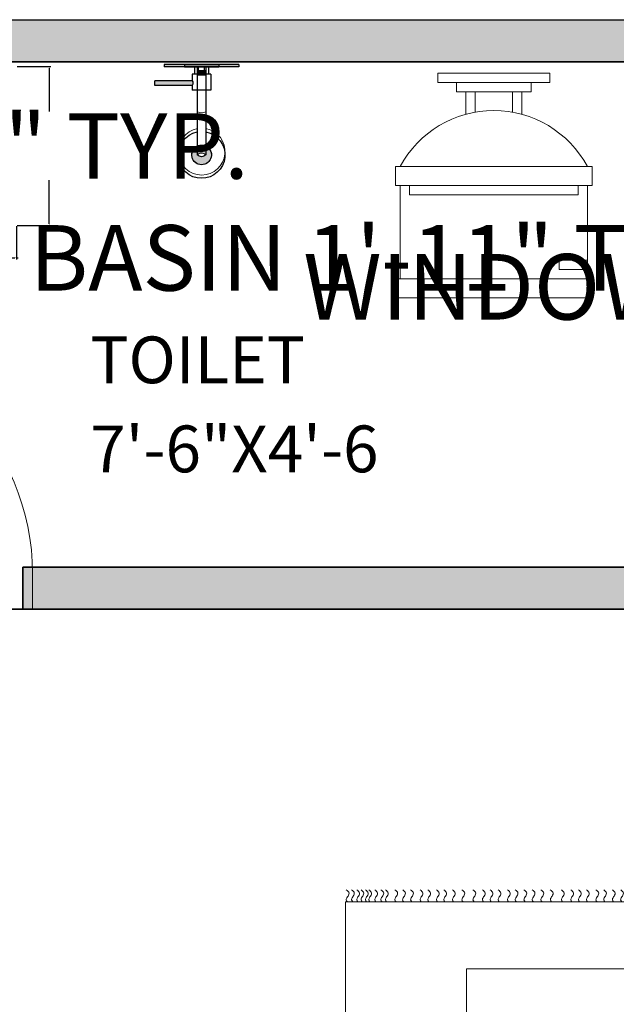
# Model space of a CAD drawing. Units: inches. Extents: x 0 to 4258, y 0 to 3769.
# Tile 22 of 30: x 3708 to 3772, y 3552 to 3657. Entities that reach past the tile are written whole.
import ezdxf

# ---------------------------------------------------------------- set-up
doc = ezdxf.new("R2010")
doc.units = ezdxf.units.IN
doc.header["$MEASUREMENT"] = 0
doc.layers.get('0').update_dxf_attribs({"color": 16})
for name, color, linetype, lineweight in [('A-ANNO-DIMS', 250, 'Continuous', 18), ('A-AREA-IDEN', 250, 'Continuous', 18), ('A-FLOR-FIXT', 250, 'Continuous', 18), ('A-WALL-PATT', 16, 'Continuous', 13), ('C-PROP', 150, 'Continuous', 25), ('doors', 250, 'Continuous', 18), ('furniture', 13, 'Continuous', 18), ('walls', 251, 'Continuous', 35)]:
    doc.layers.add(name, color=color, linetype=linetype, lineweight=lineweight)
doc.layers.add('PLUMBING FIXTURES', color=250, linetype='Continuous')
doc.styles.get("Standard").update_dxf_attribs({"font": 'arial.ttf'})
doc.dimstyles.get("Standard").update_dxf_attribs({"dimtxt": 7, "dimasz": 0.18, "dimexe": 0.18, "dimexo": 0.0625, "dimgap": 0.09, "dimtad": 0, "dimtih": 1, "dimtoh": 1, "dimzin": 0, "dimdsep": 46, "dimlunit": 3, "dimtxsty": 'Standard', "dimcen": 0.09, "dimadec": 0, "dimazin": 0, "dimtfac": 1, "dimtofl": 0, "dimtmove": 0, "dimatfit": 3, "dimfxl": 1, "dimtolj": 1, "dimtzin": 0, "dimarcsym": 0})

# ---------------------------------------------------------------- blocks, each defined once
blk = doc.blocks.new('CARPET')
at = {"layer": 'furniture'}
for p, q in [((-51.53, -98.11), (-51.53, -55.12)), ((-51.53, -55.12), (-41.27, -55.12)), ((36, -55.12), (51.55, -55.12)), ((51.55, -55.12), (51.55, -98.11)), ((51.55, -98.11), (-51.53, -98.11))]:
    blk.add_line(p, q, dxfattribs=at)
for points, knots in [([(-53.37, -55.99), (-53.22, -55.8), (-52.9, -55.41), (-52.34, -55.8), (-51.89, -56.08), (-51.65, -55.91), (-51.53, -55.83)], [0, 0, 0, 0, 0.653278, 1.290138, 1.740457, 2.114451, 2.114451, 2.114451, 2.114451]), ([(53.37, -55.99), (53.22, -55.8), (52.9, -55.41), (52.34, -55.8), (51.89, -56.08), (51.65, -55.91), (51.53, -55.83)], [0, 0, 0, 0, 0.653278, 1.290138, 1.740457, 2.114451, 2.114451, 2.114451, 2.114451]), ([(-53.37, -57.26), (-53.22, -57.07), (-52.9, -56.67), (-52.34, -57.07), (-51.89, -57.35), (-51.65, -57.17), (-51.53, -57.1)], [0, 0, 0, 0, 0.653278, 1.290138, 1.740457, 2.114451, 2.114451, 2.114451, 2.114451]), ([(53.37, -57.26), (53.22, -57.07), (52.9, -56.67), (52.34, -57.07), (51.89, -57.35), (51.65, -57.17), (51.53, -57.1)], [0, 0, 0, 0, 0.653278, 1.290138, 1.740457, 2.114451, 2.114451, 2.114451, 2.114451]), ([(-53.37, -58.59), (-53.22, -58.4), (-52.9, -58.01), (-52.34, -58.4), (-51.89, -58.68), (-51.65, -58.5), (-51.53, -58.43)], [0, 0, 0, 0, 0.653278, 1.290138, 1.740457, 2.114451, 2.114451, 2.114451, 2.114451]), ([(53.37, -58.59), (53.22, -58.4), (52.9, -58.01), (52.34, -58.4), (51.89, -58.68), (51.65, -58.5), (51.53, -58.43)], [0, 0, 0, 0, 0.653278, 1.290138, 1.740457, 2.114451, 2.114451, 2.114451, 2.114451]), ([(-53.37, -59.78), (-53.22, -59.58), (-52.9, -59.19), (-52.34, -59.58), (-51.89, -59.86), (-51.65, -59.69), (-51.53, -59.61)], [0, 0, 0, 0, 0.653278, 1.290138, 1.740457, 2.114451, 2.114451, 2.114451, 2.114451]), ([(53.37, -59.78), (53.22, -59.58), (52.9, -59.19), (52.34, -59.58), (51.89, -59.86), (51.65, -59.69), (51.53, -59.61)], [0, 0, 0, 0, 0.653278, 1.290138, 1.740457, 2.114451, 2.114451, 2.114451, 2.114451]), ([(-53.37, -61.22), (-53.22, -61.02), (-52.9, -60.63), (-52.34, -61.02), (-51.89, -61.3), (-51.65, -61.13), (-51.53, -61.05)], [0, 0, 0, 0, 0.653278, 1.290138, 1.740457, 2.114451, 2.114451, 2.114451, 2.114451]), ([(53.37, -61.22), (53.22, -61.02), (52.9, -60.63), (52.34, -61.02), (51.89, -61.3), (51.65, -61.13), (51.53, -61.05)], [0, 0, 0, 0, 0.653278, 1.290138, 1.740457, 2.114451, 2.114451, 2.114451, 2.114451]), ([(-53.37, -62.44), (-53.22, -62.25), (-52.9, -61.86), (-52.34, -62.25), (-51.89, -62.53), (-51.65, -62.36), (-51.53, -62.28)], [0, 0, 0, 0, 0.653278, 1.290138, 1.740457, 2.114451, 2.114451, 2.114451, 2.114451]), ([(-53.37, -63.63), (-53.22, -63.43), (-52.9, -63.04), (-52.34, -63.43), (-51.89, -63.72), (-51.65, -63.54), (-51.53, -63.46)], [0, 0, 0, 0, 0.653278, 1.290138, 1.740457, 2.114451, 2.114451, 2.114451, 2.114451]), ([(53.37, -62.44), (53.22, -62.25), (52.9, -61.86), (52.34, -62.25), (51.89, -62.53), (51.65, -62.36), (51.53, -62.28)], [0, 0, 0, 0, 0.653278, 1.290138, 1.740457, 2.114451, 2.114451, 2.114451, 2.114451]), ([(53.37, -63.63), (53.22, -63.43), (52.9, -63.04), (52.34, -63.43), (51.89, -63.72), (51.65, -63.54), (51.53, -63.46)], [0, 0, 0, 0, 0.653278, 1.290138, 1.740457, 2.114451, 2.114451, 2.114451, 2.114451]), ([(-53.37, -65.07), (-53.22, -64.87), (-52.9, -64.48), (-52.34, -64.87), (-51.89, -65.15), (-51.65, -64.98), (-51.53, -64.9)], [0, 0, 0, 0, 0.653278, 1.290138, 1.740457, 2.114451, 2.114451, 2.114451, 2.114451]), ([(53.37, -65.07), (53.22, -64.87), (52.9, -64.48), (52.34, -64.87), (51.89, -65.15), (51.65, -64.98), (51.53, -64.9)], [0, 0, 0, 0, 0.653278, 1.290138, 1.740457, 2.114451, 2.114451, 2.114451, 2.114451]), ([(-53.37, -66.76), (-53.22, -66.56), (-52.9, -66.17), (-52.34, -66.56), (-51.89, -66.84), (-51.65, -66.67), (-51.53, -66.59)], [0, 0, 0, 0, 0.653278, 1.290138, 1.740457, 2.114451, 2.114451, 2.114451, 2.114451]), ([(-53.37, -68.2), (-53.22, -68), (-52.9, -67.61), (-52.34, -68), (-51.89, -68.28), (-51.65, -68.11), (-51.53, -68.03)], [0, 0, 0, 0, 0.653278, 1.290138, 1.740457, 2.114451, 2.114451, 2.114451, 2.114451]), ([(53.37, -66.76), (53.22, -66.56), (52.9, -66.17), (52.34, -66.56), (51.89, -66.84), (51.65, -66.67), (51.53, -66.59)], [0, 0, 0, 0, 0.653278, 1.290138, 1.740457, 2.114451, 2.114451, 2.114451, 2.114451]), ([(53.37, -68.2), (53.22, -68), (52.9, -67.61), (52.34, -68), (51.89, -68.28), (51.65, -68.11), (51.53, -68.03)], [0, 0, 0, 0, 0.653278, 1.290138, 1.740457, 2.114451, 2.114451, 2.114451, 2.114451]), ([(-53.37, -69.53), (-53.22, -69.33), (-52.9, -68.94), (-52.34, -69.33), (-51.89, -69.61), (-51.65, -69.44), (-51.53, -69.36)], [0, 0, 0, 0, 0.653278, 1.290138, 1.740457, 2.114451, 2.114451, 2.114451, 2.114451]), ([(53.37, -69.53), (53.22, -69.33), (52.9, -68.94), (52.34, -69.33), (51.89, -69.61), (51.65, -69.44), (51.53, -69.36)], [0, 0, 0, 0, 0.653278, 1.290138, 1.740457, 2.114451, 2.114451, 2.114451, 2.114451]), ([(-53.37, -70.79), (-53.22, -70.6), (-52.9, -70.21), (-52.34, -70.6), (-51.89, -70.88), (-51.65, -70.7), (-51.53, -70.63)], [0, 0, 0, 0, 0.653278, 1.290138, 1.740457, 2.114451, 2.114451, 2.114451, 2.114451]), ([(53.37, -70.79), (53.22, -70.6), (52.9, -70.21), (52.34, -70.6), (51.89, -70.88), (51.65, -70.7), (51.53, -70.63)], [0, 0, 0, 0, 0.653278, 1.290138, 1.740457, 2.114451, 2.114451, 2.114451, 2.114451]), ([(-53.37, -72.12), (-53.22, -71.93), (-52.9, -71.54), (-52.34, -71.93), (-51.89, -72.21), (-51.65, -72.04), (-51.53, -71.96)], [0, 0, 0, 0, 0.653278, 1.290138, 1.740457, 2.114451, 2.114451, 2.114451, 2.114451]), ([(53.37, -72.12), (53.22, -71.93), (52.9, -71.54), (52.34, -71.93), (51.89, -72.21), (51.65, -72.04), (51.53, -71.96)], [0, 0, 0, 0, 0.653278, 1.290138, 1.740457, 2.114451, 2.114451, 2.114451, 2.114451]), ([(-53.37, -73.31), (-53.22, -73.11), (-52.9, -72.72), (-52.34, -73.11), (-51.89, -73.4), (-51.65, -73.22), (-51.53, -73.14)], [0, 0, 0, 0, 0.653278, 1.290138, 1.740457, 2.114451, 2.114451, 2.114451, 2.114451]), ([(53.37, -73.31), (53.22, -73.11), (52.9, -72.72), (52.34, -73.11), (51.89, -73.4), (51.65, -73.22), (51.53, -73.14)], [0, 0, 0, 0, 0.653278, 1.290138, 1.740457, 2.114451, 2.114451, 2.114451, 2.114451]), ([(-53.37, -74.75), (-53.22, -74.55), (-52.9, -74.16), (-52.34, -74.55), (-51.89, -74.83), (-51.65, -74.66), (-51.53, -74.58)], [0, 0, 0, 0, 0.653278, 1.290138, 1.740457, 2.114451, 2.114451, 2.114451, 2.114451]), ([(53.37, -74.75), (53.22, -74.55), (52.9, -74.16), (52.34, -74.55), (51.89, -74.83), (51.65, -74.66), (51.53, -74.58)], [0, 0, 0, 0, 0.653278, 1.290138, 1.740457, 2.114451, 2.114451, 2.114451, 2.114451]), ([(-53.37, -75.98), (-53.22, -75.78), (-52.9, -75.39), (-52.34, -75.78), (-51.89, -76.06), (-51.65, -75.89), (-51.53, -75.81)], [0, 0, 0, 0, 0.653278, 1.290138, 1.740457, 2.114451, 2.114451, 2.114451, 2.114451]), ([(-53.37, -77.16), (-53.22, -76.96), (-52.9, -76.57), (-52.34, -76.96), (-51.89, -77.25), (-51.65, -77.07), (-51.53, -76.99)], [0, 0, 0, 0, 0.653278, 1.290138, 1.740457, 2.114451, 2.114451, 2.114451, 2.114451]), ([(53.37, -75.98), (53.22, -75.78), (52.9, -75.39), (52.34, -75.78), (51.89, -76.06), (51.65, -75.89), (51.53, -75.81)], [0, 0, 0, 0, 0.653278, 1.290138, 1.740457, 2.114451, 2.114451, 2.114451, 2.114451]), ([(53.37, -77.16), (53.22, -76.96), (52.9, -76.57), (52.34, -76.96), (51.89, -77.25), (51.65, -77.07), (51.53, -76.99)], [0, 0, 0, 0, 0.653278, 1.290138, 1.740457, 2.114451, 2.114451, 2.114451, 2.114451]), ([(-53.37, -78.6), (-53.22, -78.4), (-52.9, -78.01), (-52.34, -78.4), (-51.89, -78.68), (-51.65, -78.51), (-51.53, -78.43)], [0, 0, 0, 0, 0.653278, 1.290138, 1.740457, 2.114451, 2.114451, 2.114451, 2.114451]), ([(53.37, -78.6), (53.22, -78.4), (52.9, -78.01), (52.34, -78.4), (51.89, -78.68), (51.65, -78.51), (51.53, -78.43)], [0, 0, 0, 0, 0.653278, 1.290138, 1.740457, 2.114451, 2.114451, 2.114451, 2.114451]), ([(-53.37, -80.29), (-53.22, -80.09), (-52.9, -79.7), (-52.34, -80.09), (-51.89, -80.37), (-51.65, -80.2), (-51.53, -80.12)], [0, 0, 0, 0, 0.653278, 1.290138, 1.740457, 2.114451, 2.114451, 2.114451, 2.114451]), ([(-53.37, -81.73), (-53.22, -81.53), (-52.9, -81.14), (-52.34, -81.53), (-51.89, -81.81), (-51.65, -81.64), (-51.53, -81.56)], [0, 0, 0, 0, 0.653278, 1.290138, 1.740457, 2.114451, 2.114451, 2.114451, 2.114451]), ([(53.37, -80.29), (53.22, -80.09), (52.9, -79.7), (52.34, -80.09), (51.89, -80.37), (51.65, -80.2), (51.53, -80.12)], [0, 0, 0, 0, 0.653278, 1.290138, 1.740457, 2.114451, 2.114451, 2.114451, 2.114451]), ([(53.37, -81.73), (53.22, -81.53), (52.9, -81.14), (52.34, -81.53), (51.89, -81.81), (51.65, -81.64), (51.53, -81.56)], [0, 0, 0, 0, 0.653278, 1.290138, 1.740457, 2.114451, 2.114451, 2.114451, 2.114451]), ([(-53.37, -83.06), (-53.22, -82.86), (-52.9, -82.47), (-52.34, -82.86), (-51.89, -83.14), (-51.65, -82.97), (-51.53, -82.89)], [0, 0, 0, 0, 0.653278, 1.290138, 1.740457, 2.114451, 2.114451, 2.114451, 2.114451]), ([(53.37, -83.06), (53.22, -82.86), (52.9, -82.47), (52.34, -82.86), (51.89, -83.14), (51.65, -82.97), (51.53, -82.89)], [0, 0, 0, 0, 0.653278, 1.290138, 1.740457, 2.114451, 2.114451, 2.114451, 2.114451]), ([(-53.37, -84.18), (-53.22, -83.99), (-52.9, -83.6), (-52.34, -83.99), (-51.89, -84.27), (-51.65, -84.09), (-51.53, -84.02)], [0, 0, 0, 0, 0.653278, 1.290138, 1.740457, 2.114451, 2.114451, 2.114451, 2.114451]), ([(53.37, -84.18), (53.22, -83.99), (52.9, -83.6), (52.34, -83.99), (51.89, -84.27), (51.65, -84.09), (51.53, -84.02)], [0, 0, 0, 0, 0.653278, 1.290138, 1.740457, 2.114451, 2.114451, 2.114451, 2.114451]), ([(-53.37, -85.51), (-53.22, -85.32), (-52.9, -84.93), (-52.34, -85.32), (-51.89, -85.6), (-51.65, -85.42), (-51.53, -85.35)], [0, 0, 0, 0, 0.653278, 1.290138, 1.740457, 2.114451, 2.114451, 2.114451, 2.114451]), ([(53.37, -85.51), (53.22, -85.32), (52.9, -84.93), (52.34, -85.32), (51.89, -85.6), (51.65, -85.42), (51.53, -85.35)], [0, 0, 0, 0, 0.653278, 1.290138, 1.740457, 2.114451, 2.114451, 2.114451, 2.114451]), ([(-53.37, -86.7), (-53.22, -86.5), (-52.9, -86.11), (-52.34, -86.5), (-51.89, -86.78), (-51.65, -86.61), (-51.53, -86.53)], [0, 0, 0, 0, 0.653278, 1.290138, 1.740457, 2.114451, 2.114451, 2.114451, 2.114451]), ([(53.37, -86.7), (53.22, -86.5), (52.9, -86.11), (52.34, -86.5), (51.89, -86.78), (51.65, -86.61), (51.53, -86.53)], [0, 0, 0, 0, 0.653278, 1.290138, 1.740457, 2.114451, 2.114451, 2.114451, 2.114451]), ([(-53.37, -88.14), (-53.22, -87.94), (-52.9, -87.55), (-52.34, -87.94), (-51.89, -88.22), (-51.65, -88.05), (-51.53, -87.97)], [0, 0, 0, 0, 0.653278, 1.290138, 1.740457, 2.114451, 2.114451, 2.114451, 2.114451]), ([(53.37, -88.14), (53.22, -87.94), (52.9, -87.55), (52.34, -87.94), (51.89, -88.22), (51.65, -88.05), (51.53, -87.97)], [0, 0, 0, 0, 0.653278, 1.290138, 1.740457, 2.114451, 2.114451, 2.114451, 2.114451]), ([(-53.37, -89.36), (-53.22, -89.17), (-52.9, -88.78), (-52.34, -89.17), (-51.89, -89.45), (-51.65, -89.28), (-51.53, -89.2)], [0, 0, 0, 0, 0.653278, 1.290138, 1.740457, 2.114451, 2.114451, 2.114451, 2.114451]), ([(-53.37, -90.55), (-53.22, -90.35), (-52.9, -89.96), (-52.34, -90.35), (-51.89, -90.64), (-51.65, -90.46), (-51.53, -90.38)], [0, 0, 0, 0, 0.653278, 1.290138, 1.740457, 2.114451, 2.114451, 2.114451, 2.114451]), ([(53.37, -89.36), (53.22, -89.17), (52.9, -88.78), (52.34, -89.17), (51.89, -89.45), (51.65, -89.28), (51.53, -89.2)], [0, 0, 0, 0, 0.653278, 1.290138, 1.740457, 2.114451, 2.114451, 2.114451, 2.114451]), ([(53.37, -90.55), (53.22, -90.35), (52.9, -89.96), (52.34, -90.35), (51.9, -90.63), (51.66, -90.47), (51.55, -90.4)], [0, 0, 0, 0, 0.653278, 1.290138, 1.740457, 2.0926, 2.0926, 2.0926, 2.0926]), ([(-53.37, -91.99), (-53.22, -91.79), (-52.9, -91.4), (-52.34, -91.79), (-51.89, -92.07), (-51.65, -91.9), (-51.53, -91.82)], [0, 0, 0, 0, 0.653278, 1.290138, 1.740457, 2.114451, 2.114451, 2.114451, 2.114451]), ([(53.37, -91.99), (53.22, -91.79), (52.9, -91.4), (52.34, -91.79), (51.9, -92.07), (51.66, -91.91), (51.55, -91.83)], [0, 0, 0, 0, 0.653278, 1.290138, 1.740457, 2.0926, 2.0926, 2.0926, 2.0926]), ([(-53.37, -92.69), (-53.22, -92.48), (-52.9, -92.08), (-52.35, -92.49), (-51.89, -92.77), (-51.65, -92.6), (-51.53, -92.52)], [0, 0, 0, 0, 0.663904, 1.307406, 1.757725, 2.131719, 2.131719, 2.131719, 2.131719]), ([(-53.37, -93.61), (-53.22, -93.42), (-52.9, -93.03), (-52.34, -93.42), (-51.89, -93.7), (-51.65, -93.52), (-51.53, -93.45)], [0, 0, 0, 0, 0.653278, 1.290138, 1.740457, 2.114451, 2.114451, 2.114451, 2.114451]), ([(53.37, -92.69), (53.22, -92.49), (52.9, -92.09), (52.34, -92.49), (51.9, -92.77), (51.66, -92.61), (51.55, -92.53)], [0, 0, 0, 0, 0.656792, 1.295826, 1.746145, 2.098292, 2.098292, 2.098292, 2.098292]), ([(53.37, -93.66), (53.22, -93.46), (52.9, -93.07), (52.34, -93.46), (51.9, -93.74), (51.66, -93.58), (51.55, -93.5)], [0, 0, 0, 0, 0.653278, 1.290138, 1.740457, 2.0926, 2.0926, 2.0926, 2.0926]), ([(-53.37, -94.55), (-53.22, -94.35), (-52.9, -93.96), (-52.34, -94.35), (-51.89, -94.63), (-51.65, -94.46), (-51.53, -94.38)], [0, 0, 0, 0, 0.653278, 1.290138, 1.740457, 2.114451, 2.114451, 2.114451, 2.114451]), ([(-53.37, -95.05), (-53.22, -94.85), (-52.9, -94.46), (-52.34, -94.85), (-51.89, -95.14), (-51.65, -94.96), (-51.53, -94.88)], [0, 0, 0, 0, 0.653278, 1.290138, 1.740457, 2.114451, 2.114451, 2.114451, 2.114451]), ([(53.37, -94.59), (53.22, -94.4), (52.9, -94.01), (52.34, -94.4), (51.9, -94.68), (51.66, -94.51), (51.55, -94.44)], [0, 0, 0, 0, 0.653278, 1.290138, 1.740457, 2.0926, 2.0926, 2.0926, 2.0926]), ([(53.37, -95.1), (53.22, -94.9), (52.9, -94.51), (52.34, -94.9), (51.9, -95.18), (51.66, -95.02), (51.55, -94.94)], [0, 0, 0, 0, 0.653278, 1.290138, 1.740457, 2.0926, 2.0926, 2.0926, 2.0926]), ([(-53.37, -95.73), (-53.22, -95.54), (-52.9, -95.15), (-52.34, -95.54), (-51.89, -95.82), (-51.65, -95.65), (-51.53, -95.57)], [0, 0, 0, 0, 0.653278, 1.290138, 1.740457, 2.114451, 2.114451, 2.114451, 2.114451]), ([(-53.37, -96.38), (-53.22, -96.18), (-52.9, -95.79), (-52.34, -96.18), (-51.89, -96.47), (-51.65, -96.29), (-51.53, -96.21)], [0, 0, 0, 0, 0.653278, 1.290138, 1.740457, 2.114451, 2.114451, 2.114451, 2.114451]), ([(53.37, -95.78), (53.22, -95.58), (52.9, -95.19), (52.34, -95.58), (51.89, -95.86), (51.65, -95.69), (51.53, -95.61)], [0, 0, 0, 0, 0.653278, 1.290138, 1.740457, 2.114451, 2.114451, 2.114451, 2.114451]), ([(53.37, -96.43), (53.22, -96.23), (52.9, -95.84), (52.34, -96.23), (51.89, -96.51), (51.65, -96.34), (51.53, -96.26)], [0, 0, 0, 0, 0.653278, 1.290138, 1.740457, 2.114451, 2.114451, 2.114451, 2.114451]), ([(-53.37, -97.17), (-53.22, -96.98), (-52.9, -96.59), (-52.34, -96.98), (-51.89, -97.26), (-51.65, -97.08), (-51.53, -97.01)], [0, 0, 0, 0, 0.653278, 1.290138, 1.740457, 2.114451, 2.114451, 2.114451, 2.114451]), ([(-53.37, -97.99), (-53.22, -97.79), (-52.9, -97.4), (-52.34, -97.79), (-51.89, -98.08), (-51.65, -97.9), (-51.53, -97.82)], [0, 0, 0, 0, 0.653278, 1.290138, 1.740457, 2.114451, 2.114451, 2.114451, 2.114451]), ([(53.37, -97.22), (53.22, -97.02), (52.9, -96.63), (52.34, -97.02), (51.89, -97.3), (51.65, -97.13), (51.53, -97.05)], [0, 0, 0, 0, 0.653278, 1.290138, 1.740457, 2.114451, 2.114451, 2.114451, 2.114451]), ([(53.37, -97.99), (53.22, -97.79), (52.9, -97.4), (52.34, -97.79), (51.89, -98.08), (51.65, -97.9), (51.53, -97.82)], [0, 0, 0, 0, 0.653278, 1.290138, 1.740457, 2.114451, 2.114451, 2.114451, 2.114451])]:
    blk.add_open_spline(points, degree=3, knots=knots, dxfattribs=at)
blk = doc.blocks.new('A$C58D270C6')
at = {"layer": 'furniture'}
for p, q in [((9.09, 124.13), (9.09, 108.87)), ((1.46, 116.5), (16.73, 116.5)), ((14.97, 94.84), (24.62, 107.92)), ((24.62, 94.93), (24.62, 107.92)), ((42.08, 108), (42.08, 36)), ((14.97, 94.93), (24.62, 94.93)), ((14.97, 94.84), (14.97, 36)), ((16.22, 94.93), (16.22, 36)), ((9.25, 36), (9.25, 20.74)), ((1.62, 28.37), (16.88, 28.37))]:
    blk.add_line(p, q, dxfattribs=at)
for points in [[(18.5, 108), (18.34, 124.13), (-0.16, 124.13), (0, 108)], [(0, 108), (77.91, 108), (77.91, 36), (0, 36)], [(4.09, 94.93), (14.97, 94.93), (14.97, 73.83), (4.09, 73.83)], [(4.09, 65.23), (14.97, 65.23), (14.97, 44.13), (4.09, 44.13)], [(18.65, 19.87), (18.5, 36), (0, 36), (0.16, 19.87)]]:
    blk.add_lwpolyline(points, close=True, dxfattribs=at)
for centre in [(9.09, 116.5), (9.25, 28.37)]:
    blk.add_circle(centre, 5.95, dxfattribs=at)
at = {"layer": 'furniture', "xscale": 0.9312884925094044, "yscale": 0.9312884925094044, "zscale": 0.9312884925094044, "rotation": 90}
blk.add_blockref('CARPET', (3.79, 74.47), dxfattribs=at)
blk = doc.blocks.new('*U18')
for p, q in [((-10, 22), (-10, 12)), ((10, 12), (10, 22)), ((-10, 21), (-7, 21)), ((-7, 20), (-10, 20)), ((-7, 21), (-7, 20)), ((9, 13), (-9, 13)), ((-9, 13), (-9, 12)), ((9, 12), (9, 13)), ((10.5, 12), (-10.5, 12)), ((-10.5, 10), (-10.5, 12)), ((10.5, 12), (10.5, 10)), ((10.5, 10), (-10.5, 10)), ((-3, 4.4065), (-3, 2)), ((3, 2), (3, 4.4065)), ((-2, 2), (-2, 4.1658)), ((2, 4.1658), (2, 2)), ((4, 2), (-4, 2)), ((-4, 2), (-4, 1)), ((4, 1), (4, 2))]:
    blk.add_line(p, q)
for points in [[(10.5, 22), (10.5, 24), (-10.5, 24), (-10.5, 22)], [(6, 0), (6, 1), (-6, 1), (-6, 0)]]:
    blk.add_lwpolyline(points, close=True)
blk.add_arc((0, 15.3333), 11.3333, 208.0725, 331.9275)
blk = doc.blocks.new('*U23')
for p, q in [((0, 0), (0, -6)), ((40, 0), (40, -6))]:
    blk.add_line(p, q)
blk.add_lwpolyline([(0, 0), (0, 40), (1.75, 40), (1.75, 0)], close=True)
blk.add_arc((0, 0), 40, 0, 90)
blk = doc.blocks.new('O.H SHOWER-PL')
at = {"layer": 'PLUMBING FIXTURES'}
for points in [[(-1.84, 0), (-1.84, -0.25), (1.84, -0.25), (1.84, 0)], [(0.46, -8.72), (0.46, -9.67, -0.422337), (-0.46, -9.67), (-0.46, -8.72, 4.325472)]]:
    blk.add_hatch(color=256, dxfattribs=at).paths.add_polyline_path(points)
for p, q in [((-1.84, 0), (-1.84, -0.25)), ((1.84, 0), (-1.84, 0)), ((1.84, 0), (1.84, -0.25)), ((1.84, -0.25), (-1.84, -0.25)), ((-0.46, -0.25), (-0.46, -9.67)), ((0.46, -0.25), (0.46, -9.67))]:
    blk.add_line(p, q, dxfattribs=at)
for centre, radius, start, end in [((0, -4.48), 1.03, 243.53, 296.47), ((0, -9.67), 2.5, 100.61, 79.39), ((0, -9.67), 1.05, 116.0349, 63.9652), ((0, -9.22), 0.643, 224.2078, 315.7922)]:
    blk.add_arc(centre, radius, start, end, dxfattribs=at)
blk = doc.blocks.new('DIVERTER-PL')
at = {"layer": 'PLUMBING FIXTURES'}
for points in [[(4, 0), (-4, 0), (-4, -0.25), (4, -0.25)], [(0.38, -1.14), (0.38, -0.7), (-0.37, -0.7), (-0.37, -1.14)], [(1, -1.75, 0.30818), (1, -2.25), (5, -2.25), (5, -1.75)]]:
    blk.add_hatch(color=256, dxfattribs=at).paths.add_polyline_path(points)
for p, q in [((-4, 0), (-4, -0.25)), ((-4, 0), (4, 0)), ((4, 0), (4, -0.25)), ((-4, -0.25), (4, -0.25)), ((-4, -0.25), (4, -0.25)), ((-1, -1.05), (-0.37, -1.05)), ((-1, -1.05), (-1, -2.75)), ((-0.75, -0.25), (-0.75, -1.05)), ((-0.37, -0.7), (0.38, -0.7)), ((-0.37, -0.7), (-0.37, -1.14)), ((-0.32, -0.7), (-0.32, -0.25)), ((0.32, -0.7), (0.32, -0.25)), ((0.38, -0.7), (0.38, -1.14)), ((0.38, -1.05), (1, -1.05)), ((0.75, -0.25), (0.75, -1.05)), ((1, -1.05), (1, -1.75)), ((-0.37, -1.14), (0.38, -1.14)), ((-1, -2.75), (1, -2.75)), ((1, -2.25), (1, -2.75))]:
    blk.add_line(p, q, dxfattribs=at)
at = {"layer": 'PLUMBING FIXTURES', "ltscale": 12}
for p, q in [((1, -1.75), (5, -1.75)), ((5, -2.25), (5, -1.75)), ((1, -2.25), (5, -2.25))]:
    blk.add_line(p, q, dxfattribs=at)
at = {"layer": 'PLUMBING FIXTURES'}
blk.add_arc((1.37, -2), 0.444, 145.7435, 214.2565, dxfattribs=at)
blk = doc.blocks.new('A$C7F153053')
at = {"layer": 'PLUMBING FIXTURES', "xscale": -1, "rotation": 270}
for name in ['DIVERTER-PL', 'O.H SHOWER-PL']:
    blk.add_blockref(name, (12.17, 4), dxfattribs=at)
blk = doc.blocks.new('SHOWER-WALL-SET')
blk.add_hatch(color=256).paths.add_polyline_path([(5.46, 1.56), (5.46, 2.5, 0.422337), (4.54, 2.5), (4.54, 1.56, -4.325472)])
blk.add_hatch(color=256).paths.add_polyline_path([(5.46, 1.56), (5.46, 2.5, 0.422337), (4.54, 2.5), (4.54, 1.56, -4.325472)])
blk.add_hatch(color=256).paths.add_polyline_path([(5.46, 1.56), (5.46, 2.5, 0.422337), (4.54, 2.5), (4.54, 1.56, -4.325472)])
blk.add_hatch(color=256).paths.add_polyline_path([(5.46, 1.56), (5.46, 2.5, 0.422337), (4.54, 2.5), (4.54, 1.56, -4.325472)])
blk.add_hatch(color=256).paths.add_polyline_path([(5.46, 1.56), (5.46, 2.5, 0.422337), (4.54, 2.5), (4.54, 1.56, -4.325472)])
blk.add_hatch(color=256).paths.add_polyline_path([(5.46, 1.56), (5.46, 2.5, 0.422337), (4.54, 2.5), (4.54, 1.56, -4.325472)])
blk.add_hatch(color=256).paths.add_polyline_path([(5.46, 1.56), (5.46, 2.5, 0.422337), (4.54, 2.5), (4.54, 1.56, -4.325472)])
blk.add_hatch(color=256).paths.add_polyline_path([(5.46, 1.56), (5.46, 2.5, 0.422337), (4.54, 2.5), (4.54, 1.56, -4.325472)])
blk.add_hatch(color=256).paths.add_polyline_path([(5.46, 1.56), (5.46, 2.5, 0.422337), (4.54, 2.5), (4.54, 1.56, -4.325472)])
blk.add_hatch(color=256).paths.add_polyline_path([(5.46, 1.56), (5.46, 2.5, 0.422337), (4.54, 2.5), (4.54, 1.56, -4.325472)])
blk.add_hatch(color=256).paths.add_polyline_path([(5.46, 1.56), (5.46, 2.5, 0.422337), (4.54, 2.5), (4.54, 1.56, -4.325472)])
blk.add_hatch(color=256).paths.add_polyline_path([(5.46, 1.56), (5.46, 2.5, 0.422337), (4.54, 2.5), (4.54, 1.56, -4.325472)])
blk.add_hatch(color=256).paths.add_polyline_path([(5.46, 1.56), (5.46, 2.5, 0.422337), (4.54, 2.5), (4.54, 1.56, -4.325472)])
blk.add_hatch(color=256).paths.add_polyline_path([(5.46, 1.56), (5.46, 2.5, 0.422337), (4.54, 2.5), (4.54, 1.56, -4.325472)])
blk.add_hatch(color=256).paths.add_polyline_path([(5.46, 1.56), (5.46, 2.5, 0.422337), (4.54, 2.5), (4.54, 1.56, -4.325472)])
blk.add_hatch(color=256).paths.add_polyline_path([(5.46, 1.56), (5.46, 2.5, 0.422337), (4.54, 2.5), (4.54, 1.56, -4.325472)])
blk.add_hatch(color=256).paths.add_polyline_path([(5.46, 1.56), (5.46, 2.5, 0.422337), (4.54, 2.5), (4.54, 1.56, -4.325472)])
blk.add_hatch(color=256).paths.add_polyline_path([(5.46, 1.56), (5.46, 2.5, 0.422337), (4.54, 2.5), (4.54, 1.56, -4.325472)])
blk.add_hatch(color=256).paths.add_polyline_path([(5.46, 1.56), (5.46, 2.5, 0.422337), (4.54, 2.5), (4.54, 1.56, -4.325472)])
blk.add_hatch(color=256).paths.add_polyline_path([(5.46, 1.56), (5.46, 2.5, 0.422337), (4.54, 2.5), (4.54, 1.56, -4.325472)])
blk.add_hatch(color=256).paths.add_polyline_path([(5.46, 1.56), (5.46, 2.5, 0.422337), (4.54, 2.5), (4.54, 1.56, -4.325472)])
blk.add_hatch(color=256).paths.add_polyline_path([(5.46, 1.56), (5.46, 2.5, 0.422337), (4.54, 2.5), (4.54, 1.56, -4.325472)])
blk.add_hatch(color=256).paths.add_polyline_path([(5.46, 1.56), (5.46, 2.5, 0.422337), (4.54, 2.5), (4.54, 1.56, -4.325472)])
blk.add_hatch(color=256).paths.add_polyline_path([(5.46, 1.56), (5.46, 2.5, 0.422337), (4.54, 2.5), (4.54, 1.56, -4.325472)])
blk.add_hatch(color=256).paths.add_polyline_path([(5.46, 1.56), (5.46, 2.5, 0.422337), (4.54, 2.5), (4.54, 1.56, -4.325472)])
blk.add_hatch(color=256).paths.add_polyline_path([(5.46, 1.56), (5.46, 2.5, 0.422337), (4.54, 2.5), (4.54, 1.56, -4.325472)])
blk.add_hatch(color=256).paths.add_polyline_path([(5.46, 1.56), (5.46, 2.5, 0.422337), (4.54, 2.5), (4.54, 1.56, -4.325472)])
blk.add_hatch(color=256).paths.add_polyline_path([(5.46, 1.56), (5.46, 2.5, 0.422337), (4.54, 2.5), (4.54, 1.56, -4.325472)])
blk.add_hatch(color=256).paths.add_polyline_path([(5.46, 1.56), (5.46, 2.5, 0.422337), (4.54, 2.5), (4.54, 1.56, -4.325472)])
blk.add_hatch(color=256).paths.add_polyline_path([(5.46, 1.56), (5.46, 2.5, 0.422337), (4.54, 2.5), (4.54, 1.56, -4.325472)])
blk.add_hatch(color=256).paths.add_polyline_path([(5.46, 1.56), (5.46, 2.5, 0.422337), (4.54, 2.5), (4.54, 1.56, -4.325472)])
blk.add_hatch(color=256).paths.add_polyline_path([(5.46, 1.56), (5.46, 2.5, 0.422337), (4.54, 2.5), (4.54, 1.56, -4.325472)])
blk.add_hatch(color=256).paths.add_polyline_path([(5.46, 1.56), (5.46, 2.5, 0.422337), (4.54, 2.5), (4.54, 1.56, -4.325472)])
blk.add_hatch(color=256).paths.add_polyline_path([(5.46, 1.56), (5.46, 2.5, 0.422337), (4.54, 2.5), (4.54, 1.56, -4.325472)])
blk.add_hatch(color=256).paths.add_polyline_path([(5.46, 1.56), (5.46, 2.5, 0.422337), (4.54, 2.5), (4.54, 1.56, -4.325472)])
blk.add_hatch(color=256).paths.add_polyline_path([(5.46, 1.56), (5.46, 2.5, 0.422337), (4.54, 2.5), (4.54, 1.56, -4.325472)])
blk.add_hatch(color=256).paths.add_polyline_path([(5.46, 1.56), (5.46, 2.5, 0.422337), (4.54, 2.5), (4.54, 1.56, -4.325472)])
blk.add_hatch(color=256).paths.add_polyline_path([(5.46, 1.56), (5.46, 2.5, 0.422337), (4.54, 2.5), (4.54, 1.56, -4.325472)])
for p, q in [((4.54, 11.92), (4.54, 2.5)), ((4.54, 11.92), (4.54, 2.5)), ((4.54, 11.92), (4.54, 2.5)), ((4.54, 11.92), (4.54, 2.5)), ((4.54, 11.92), (4.54, 2.5)), ((4.54, 11.92), (4.54, 2.5)), ((4.54, 11.92), (4.54, 2.5)), ((4.54, 11.92), (4.54, 2.5)), ((4.54, 11.92), (4.54, 2.5)), ((4.54, 11.92), (4.54, 2.5)), ((4.54, 11.92), (4.54, 2.5)), ((4.54, 11.92), (4.54, 2.5)), ((4.54, 11.92), (4.54, 2.5)), ((4.54, 11.92), (4.54, 2.5)), ((4.54, 11.92), (4.54, 2.5)), ((4.54, 11.92), (4.54, 2.5)), ((4.54, 11.92), (4.54, 2.5)), ((4.54, 11.92), (4.54, 2.5)), ((4.54, 11.92), (4.54, 2.5)), ((4.54, 11.92), (4.54, 2.5)), ((4.54, 11.92), (4.54, 2.5)), ((4.54, 11.92), (4.54, 2.5)), ((4.54, 11.92), (4.54, 2.5)), ((4.54, 11.92), (4.54, 2.5)), ((4.54, 11.92), (4.54, 2.5)), ((4.54, 11.92), (4.54, 2.5)), ((4.54, 11.92), (4.54, 2.5)), ((4.54, 11.92), (4.54, 2.5)), ((4.54, 11.92), (4.54, 2.5)), ((4.54, 11.92), (4.54, 2.5)), ((4.54, 11.92), (4.54, 2.5)), ((4.54, 11.92), (4.54, 2.5)), ((4.54, 11.92), (4.54, 2.5)), ((4.54, 11.92), (4.54, 2.5)), ((4.54, 11.92), (4.54, 2.5)), ((4.54, 11.92), (4.54, 2.5)), ((4.54, 11.92), (4.54, 2.5)), ((4.54, 11.92), (4.54, 2.5)), ((5.46, 11.92), (5.46, 2.5)), ((5.46, 11.92), (5.46, 2.5)), ((5.46, 11.92), (5.46, 2.5)), ((5.46, 11.92), (5.46, 2.5)), ((5.46, 11.92), (5.46, 2.5)), ((5.46, 11.92), (5.46, 2.5)), ((5.46, 11.92), (5.46, 2.5)), ((5.46, 11.92), (5.46, 2.5)), ((5.46, 11.92), (5.46, 2.5)), ((5.46, 11.92), (5.46, 2.5)), ((5.46, 11.92), (5.46, 2.5)), ((5.46, 11.92), (5.46, 2.5)), ((5.46, 11.92), (5.46, 2.5)), ((5.46, 11.92), (5.46, 2.5)), ((5.46, 11.92), (5.46, 2.5)), ((5.46, 11.92), (5.46, 2.5)), ((5.46, 11.92), (5.46, 2.5)), ((5.46, 11.92), (5.46, 2.5)), ((5.46, 11.92), (5.46, 2.5)), ((5.46, 11.92), (5.46, 2.5)), ((5.46, 11.92), (5.46, 2.5)), ((5.46, 11.92), (5.46, 2.5)), ((5.46, 11.92), (5.46, 2.5)), ((5.46, 11.92), (5.46, 2.5)), ((5.46, 11.92), (5.46, 2.5)), ((5.46, 11.92), (5.46, 2.5)), ((5.46, 11.92), (5.46, 2.5)), ((5.46, 11.92), (5.46, 2.5)), ((5.46, 11.92), (5.46, 2.5)), ((5.46, 11.92), (5.46, 2.5)), ((5.46, 11.92), (5.46, 2.5)), ((5.46, 11.92), (5.46, 2.5)), ((5.46, 11.92), (5.46, 2.5)), ((5.46, 11.92), (5.46, 2.5)), ((5.46, 11.92), (5.46, 2.5)), ((5.46, 11.92), (5.46, 2.5)), ((5.46, 11.92), (5.46, 2.5)), ((5.46, 11.92), (5.46, 2.5))]:
    blk.add_line(p, q)
for centre, radius, start, end in [((5.01, 8.04), 1.03, 243.53, 296.47), ((5.01, 8.04), 1.03, 243.53, 296.47), ((5.01, 8.04), 1.03, 243.53, 296.47), ((5.01, 8.04), 1.03, 243.53, 296.47), ((5.01, 8.04), 1.03, 243.53, 296.47), ((5.01, 8.04), 1.03, 243.53, 296.47), ((5.01, 8.04), 1.03, 243.53, 296.47), ((5.01, 8.04), 1.03, 243.53, 296.47), ((5.01, 8.04), 1.03, 243.53, 296.47), ((5.01, 8.04), 1.03, 243.53, 296.47), ((5.01, 8.04), 1.03, 243.53, 296.47), ((5.01, 8.04), 1.03, 243.53, 296.47), ((5.01, 8.04), 1.03, 243.53, 296.47), ((5.01, 8.04), 1.03, 243.53, 296.47), ((5.01, 8.04), 1.03, 243.53, 296.47), ((5.01, 8.04), 1.03, 243.53, 296.47), ((5.01, 8.04), 1.03, 243.53, 296.47), ((5.01, 8.04), 1.03, 243.53, 296.47), ((5.01, 8.04), 1.03, 243.53, 296.47), ((5.01, 8.04), 1.03, 243.53, 296.47), ((5.01, 8.04), 1.03, 243.53, 296.47), ((5.01, 8.04), 1.03, 243.53, 296.47), ((5.01, 8.04), 1.03, 243.53, 296.47), ((5.01, 8.04), 1.03, 243.53, 296.47), ((5.01, 8.04), 1.03, 243.53, 296.47), ((5.01, 8.04), 1.03, 243.53, 296.47), ((5.01, 8.04), 1.03, 243.53, 296.47), ((5.01, 8.04), 1.03, 243.53, 296.47), ((5.01, 8.04), 1.03, 243.53, 296.47), ((5.01, 8.04), 1.03, 243.53, 296.47), ((5.01, 8.04), 1.03, 243.53, 296.47), ((5.01, 8.04), 1.03, 243.53, 296.47), ((5.01, 8.04), 1.03, 243.53, 296.47), ((5.01, 8.04), 1.03, 243.53, 296.47), ((5.01, 8.04), 1.03, 243.53, 296.47), ((5.01, 8.04), 1.03, 243.53, 296.47), ((5.01, 8.04), 1.03, 243.53, 296.47), ((5.01, 8.04), 1.03, 243.53, 296.47), ((5.01, 2.85), 2.5, 100.61, 79.39), ((5.01, 2.85), 2.5, 100.61, 79.39), ((5.01, 2.85), 2.5, 100.61, 79.39), ((5.01, 2.85), 2.5, 100.61, 79.39), ((5.01, 2.85), 2.5, 100.61, 79.39), ((5.01, 2.85), 2.5, 100.61, 79.39), ((5.01, 2.85), 2.5, 100.61, 79.39), ((5.01, 2.85), 2.5, 100.61, 79.39), ((5.01, 2.85), 2.5, 100.61, 79.39), ((5.01, 2.85), 2.5, 100.61, 79.39), ((5.01, 2.85), 2.5, 100.61, 79.39), ((5.01, 2.85), 2.5, 100.61, 79.39), ((5.01, 2.85), 2.5, 100.61, 79.39), ((5.01, 2.85), 2.5, 100.61, 79.39), ((5.01, 2.85), 2.5, 100.61, 79.39), ((5.01, 2.85), 2.5, 100.61, 79.39), ((5.01, 2.85), 2.5, 100.61, 79.39), ((5.01, 2.85), 2.5, 100.61, 79.39), ((5.01, 2.85), 2.5, 100.61, 79.39), ((5.01, 2.85), 2.5, 100.61, 79.39), ((5.01, 2.85), 2.5, 100.61, 79.39), ((5.01, 2.85), 2.5, 100.61, 79.39), ((5.01, 2.85), 2.5, 100.61, 79.39), ((5.01, 2.85), 2.5, 100.61, 79.39), ((5.01, 2.85), 2.5, 100.61, 79.39), ((5.01, 2.85), 2.5, 100.61, 79.39), ((5.01, 2.85), 2.5, 100.61, 79.39), ((5.01, 2.85), 2.5, 100.61, 79.39), ((5.01, 2.85), 2.5, 100.61, 79.39), ((5.01, 2.85), 2.5, 100.61, 79.39), ((5.01, 2.85), 2.5, 100.61, 79.39), ((5.01, 2.85), 2.5, 100.61, 79.39), ((5.01, 2.85), 2.5, 100.61, 79.39), ((5.01, 2.85), 2.5, 100.61, 79.39), ((5.01, 2.85), 2.5, 100.61, 79.39), ((5.01, 2.85), 2.5, 100.61, 79.39), ((5.01, 2.85), 2.5, 100.61, 79.39), ((5.01, 2.85), 2.5, 100.61, 79.39), ((5, 2.5), 1.05, 296.0348, 243.9651), ((5, 2.5), 1.05, 296.0348, 243.9651), ((5, 2.5), 1.05, 296.0348, 243.9651), ((5, 2.5), 1.05, 296.0348, 243.9651), ((5, 2.5), 1.05, 296.0348, 243.9651), ((5, 2.5), 1.05, 296.0348, 243.9651), ((5, 2.5), 1.05, 296.0348, 243.9651), ((5, 2.5), 1.05, 296.0348, 243.9651), ((5, 2.5), 1.05, 296.0348, 243.9651), ((5, 2.5), 1.05, 296.0348, 243.9651), ((5, 2.5), 1.05, 296.0348, 243.9651), ((5, 2.5), 1.05, 296.0348, 243.9651), ((5, 2.5), 1.05, 296.0348, 243.9651), ((5, 2.5), 1.05, 296.0348, 243.9651), ((5, 2.5), 1.05, 296.0348, 243.9651), ((5, 2.5), 1.05, 296.0348, 243.9651), ((5, 2.5), 1.05, 296.0348, 243.9651), ((5, 2.5), 1.05, 296.0348, 243.9651), ((5, 2.5), 1.05, 296.0348, 243.9651), ((5, 2.5), 1.05, 296.0348, 243.9651), ((5, 2.5), 1.05, 296.0348, 243.9651), ((5, 2.5), 1.05, 296.0348, 243.9651), ((5, 2.5), 1.05, 296.0348, 243.9651), ((5, 2.5), 1.05, 296.0348, 243.9651), ((5, 2.5), 1.05, 296.0348, 243.9651), ((5, 2.5), 1.05, 296.0348, 243.9651), ((5, 2.5), 1.05, 296.0348, 243.9651), ((5, 2.5), 1.05, 296.0348, 243.9651), ((5, 2.5), 1.05, 296.0348, 243.9651), ((5, 2.5), 1.05, 296.0348, 243.9651), ((5, 2.5), 1.05, 296.0348, 243.9651), ((5, 2.5), 1.05, 296.0348, 243.9651), ((5, 2.5), 1.05, 296.0348, 243.9651), ((5, 2.5), 1.05, 296.0348, 243.9651), ((5, 2.5), 1.05, 296.0348, 243.9651), ((5, 2.5), 1.05, 296.0348, 243.9651), ((5, 2.5), 1.05, 296.0348, 243.9651), ((5, 2.5), 1.05, 296.0348, 243.9651), ((5, 2.05), 0.643, 44.2078, 135.7922), ((5, 2.05), 0.643, 44.2078, 135.7922), ((5, 2.05), 0.643, 44.2078, 135.7922), ((5, 2.05), 0.643, 44.2078, 135.7922), ((5, 2.05), 0.643, 44.2078, 135.7922), ((5, 2.05), 0.643, 44.2078, 135.7922), ((5, 2.05), 0.643, 44.2078, 135.7922), ((5, 2.05), 0.643, 44.2078, 135.7922), ((5, 2.05), 0.643, 44.2078, 135.7922), ((5, 2.05), 0.643, 44.2078, 135.7922), ((5, 2.05), 0.643, 44.2078, 135.7922), ((5, 2.05), 0.643, 44.2078, 135.7922), ((5, 2.05), 0.643, 44.2078, 135.7922), ((5, 2.05), 0.643, 44.2078, 135.7922), ((5, 2.05), 0.643, 44.2078, 135.7922), ((5, 2.05), 0.643, 44.2078, 135.7922), ((5, 2.05), 0.643, 44.2078, 135.7922), ((5, 2.05), 0.643, 44.2078, 135.7922), ((5, 2.05), 0.643, 44.2078, 135.7922), ((5, 2.05), 0.643, 44.2078, 135.7922), ((5, 2.05), 0.643, 44.2078, 135.7922), ((5, 2.05), 0.643, 44.2078, 135.7922), ((5, 2.05), 0.643, 44.2078, 135.7922), ((5, 2.05), 0.643, 44.2078, 135.7922), ((5, 2.05), 0.643, 44.2078, 135.7922), ((5, 2.05), 0.643, 44.2078, 135.7922), ((5, 2.05), 0.643, 44.2078, 135.7922), ((5, 2.05), 0.643, 44.2078, 135.7922), ((5, 2.05), 0.643, 44.2078, 135.7922), ((5, 2.05), 0.643, 44.2078, 135.7922), ((5, 2.05), 0.643, 44.2078, 135.7922), ((5, 2.05), 0.643, 44.2078, 135.7922), ((5, 2.05), 0.643, 44.2078, 135.7922), ((5, 2.05), 0.643, 44.2078, 135.7922), ((5, 2.05), 0.643, 44.2078, 135.7922), ((5, 2.05), 0.643, 44.2078, 135.7922), ((5, 2.05), 0.643, 44.2078, 135.7922), ((5, 2.05), 0.643, 44.2078, 135.7922)]:
    blk.add_arc(centre, radius, start, end)
at = {"ltscale": 35, "rotation": 89.99999999999999}
blk.add_blockref('A$C7F153053', (9, 0), dxfattribs=at)
blk = doc.blocks.new('*D54')
at = {"layer": 'A-ANNO-DIMS', "color": 0, "lineweight": -2, "transparency": 16777216}
for p, q in [((3684.72, 3634.74), (3684.72, 3631.16)), ((3707.82, 3634.74), (3707.82, 3631.16)), ((3684.9, 3631.34), (3707.64, 3631.34)), ((3707.82, 3631.34), (3708, 3631.34))]:
    blk.add_line(p, q, dxfattribs=at)
at = {"layer": 'A-ANNO-DIMS', "color": 0, "transparency": 16777216}
for points in [[(3684.9, 3631.37), (3684.9, 3631.31), (3684.72, 3631.34)], [(3707.64, 3631.37), (3707.64, 3631.31), (3707.82, 3631.34)]]:
    blk.add_solid(points, dxfattribs=at)
at = {"layer": 'Defpoints', "color": 0, "transparency": 16777216}
for p in [(3684.72, 3634.8), (3707.82, 3634.8), (3707.82, 3631.34)]:
    blk.add_point(p, dxfattribs=at)
at = {"layer": 'A-ANNO-DIMS', "color": 0, "transparency": 16777216, "insert": (3748.02, 3631.34), "char_height": 7, "attachment_point": 5}
blk.add_mtext('\\A1;BASIN 1\'-11" TYP.', dxfattribs=at)
blk = doc.blocks.new('*D55')
at = {"layer": 'A-ANNO-DIMS', "color": 0, "lineweight": -2, "transparency": 16777216}
for p, q in [((3707.89, 3651.8), (3711.47, 3651.8)), ((3711.29, 3651.62), (3711.29, 3646.97)), ((3711.29, 3634.98), (3711.29, 3639.64)), ((3707.89, 3634.8), (3711.47, 3634.8))]:
    blk.add_line(p, q, dxfattribs=at)
at = {"layer": 'A-ANNO-DIMS', "color": 0, "transparency": 16777216}
for points in [[(3711.26, 3651.62), (3711.32, 3651.62), (3711.29, 3651.8)], [(3711.26, 3634.98), (3711.32, 3634.98), (3711.29, 3634.8)]]:
    blk.add_solid(points, dxfattribs=at)
at = {"layer": 'Defpoints', "color": 0, "transparency": 16777216}
for p in [(3707.82, 3651.8), (3711.29, 3651.8), (3707.82, 3634.8)]:
    blk.add_point(p, dxfattribs=at)
at = {"layer": 'A-ANNO-DIMS', "color": 0, "transparency": 16777216, "insert": (3711.29, 3643.3), "char_height": 7, "attachment_point": 5}
blk.add_mtext('\\A1;1\'-5" TYP.', dxfattribs=at)
blk = doc.blocks.new('*D62')
at = {"layer": 'A-ANNO-DIMS', "color": 0, "lineweight": -2, "transparency": 16777216}
for p, q in [((3777.87, 3638.77), (3781.14, 3638.77)), ((3780.96, 3638.59), (3780.96, 3631.96)), ((3780.96, 3617.91), (3780.96, 3624.54)), ((3777.87, 3617.73), (3781.14, 3617.73))]:
    blk.add_line(p, q, dxfattribs=at)
at = {"layer": 'A-ANNO-DIMS', "color": 0, "transparency": 16777216}
for points in [[(3780.93, 3638.59), (3780.99, 3638.59), (3780.96, 3638.77)], [(3780.93, 3617.91), (3780.99, 3617.91), (3780.96, 3617.73)]]:
    blk.add_solid(points, dxfattribs=at)
at = {"layer": 'Defpoints', "color": 0, "transparency": 16777216}
for p in [(3777.8, 3638.77), (3780.96, 3638.77), (3777.8, 3617.73)]:
    blk.add_point(p, dxfattribs=at)
at = {"layer": 'A-ANNO-DIMS', "color": 0, "transparency": 16777216, "insert": (3780.96, 3628.25), "char_height": 7, "attachment_point": 5}
blk.add_mtext('\\A1;WINDOW 1\'-9" TYP.', dxfattribs=at)

msp = doc.modelspace()

# ---------------------------------------------------------------- hatches: boundary and pattern name
at = {"layer": 'A-WALL-PATT'}
h = msp.add_hatch(color=256, dxfattribs=at)
h.dxf.hatch_style = 1
h.paths.add_polyline_path([(3753.804, 3425.793), (3753.804, 3437.642), (3815.304, 3437.642), (3815.304, 3421.293), (3819.804, 3421.293), (3819.804, 3442.142), (3749.304, 3442.142), (3749.304, 3425.793), (3683.304, 3425.793), (3683.304, 3652.293), (3773.304, 3652.293), (3773.304, 3638.769), (3777.804, 3638.769), (3777.804, 3656.793), (3678.804, 3656.793), (3678.804, 3163.293), (3711.393, 3163.293), (3711.393, 3167.793), (3683.304, 3167.793), (3683.304, 3374.793), (3693.303, 3374.793), (3693.303, 3379.293), (3683.304, 3379.293), (3683.304, 3421.293), (3749.304, 3421.293), (3749.304, 3379.293), (3741.449, 3379.293), (3741.449, 3374.793), (3753.804, 3374.793)])
h = msp.add_hatch(color=256, dxfattribs=at)
h.dxf.hatch_style = 1
h.paths.add_polyline_path([(3777.804, 3598.293), (3777.804, 3617.728), (3773.304, 3617.728), (3773.304, 3598.293), (3708.48, 3598.293), (3708.48, 3593.793), (3777.804, 3593.793)])
h = msp.add_hatch(color=256, dxfattribs=at)
h.dxf.hatch_style = 1
h.paths.add_polyline_path([(3777.804, 3598.293), (3777.804, 3617.728), (3773.304, 3617.728), (3773.304, 3598.293), (3708.48, 3598.293), (3708.48, 3593.793), (3777.804, 3593.793)])

# ---------------------------------------------------------------- linework, layer by layer
at = {"layer": 'C-PROP'}
msp.add_line((3678.804, 3656.793), (4038.804, 3656.793), dxfattribs=at)
at = {"layer": 'walls'}
for p, q in [((3683.304, 3652.293), (3773.304, 3652.293)), ((3708.47, 3598.293), (3773.304, 3598.293)), ((3708.48, 3593.793), (3708.48, 3598.293)), ((3683.304, 3593.793), (3815.304, 3593.793))]:
    msp.add_line(p, q, dxfattribs=at)

# ---------------------------------------------------------------- block references
at = {"layer": 'A-FLOR-FIXT'}
msp.add_blockref('SHOWER-WALL-SET', (3722.592, 3639.846), dxfattribs=at)
at = {"layer": 'A-FLOR-FIXT', "rotation": 180}
msp.add_blockref('*U18', (3758.835, 3651.091), dxfattribs=at)
at = {"layer": 'doors', "xscale": 0.6294121846440242, "yscale": 0.6294121846440242, "zscale": 0.6294121846440242}
msp.add_blockref('*U23', (3684.348, 3597.57), dxfattribs=at)
at = {"layer": 'furniture', "xscale": 0.7500000390647866, "yscale": 0.7500000390647866, "zscale": 0.7500000390647866, "rotation": 180}
msp.add_blockref('A$C58D270C6', (3814.348, 3582.385), dxfattribs=at)

# ---------------------------------------------------------------- texts
at = {"layer": 'A-AREA-IDEN'}
for s, p in [('TOILET', (3715.693, 3617.945)), ('7\'-6"X4\'-6', (3715.693, 3608.43))]:
    msp.add_text(s, height=5, dxfattribs=at).set_placement(p)

# ---------------------------------------------------------------- dimensions: what is measured, and where the dimension line sits
at = {"layer": 'A-ANNO-DIMS'}
for base, p1, p2, text, picture, middle in [((3711.29, 3651.803), (3707.824, 3634.804), (3707.824, 3651.803), '<> TYP.', '*D55', (3711.29, 3643.303)), ((3780.96, 3638.769), (3777.804, 3617.728), (3777.804, 3638.769), 'WINDOW <> TYP.', '*D62', (3780.96, 3628.249))]:
    dim = msp.add_linear_dim(base=base, p1=p1, p2=p2, angle=90, text=text, dimstyle='Standard', override={"dimdec": 1, "dimlfac": 1, "dimrnd": 0, "dimzin": 1, "dimdsep": 46, "dimlunit": 4, "dimfrac": 2}, dxfattribs=at)
    dim.commit()
    dim.dimension.update_dxf_attribs({"geometry": picture, "text_midpoint": middle})
dim = msp.add_linear_dim(base=(3707.824, 3631.338), p1=(3684.717, 3634.804), p2=(3707.824, 3634.804), text='BASIN <> TYP.', dimstyle='Standard', override={"dimdec": 1, "dimlfac": 1, "dimrnd": 0, "dimzin": 1, "dimdsep": 46, "dimlunit": 4, "dimfrac": 2}, dxfattribs=at)
dim.commit()
dim.dimension.update_dxf_attribs({"geometry": '*D54', "text_midpoint": (3748.024, 3631.338)})

doc.saveas('drawing.dxf')
